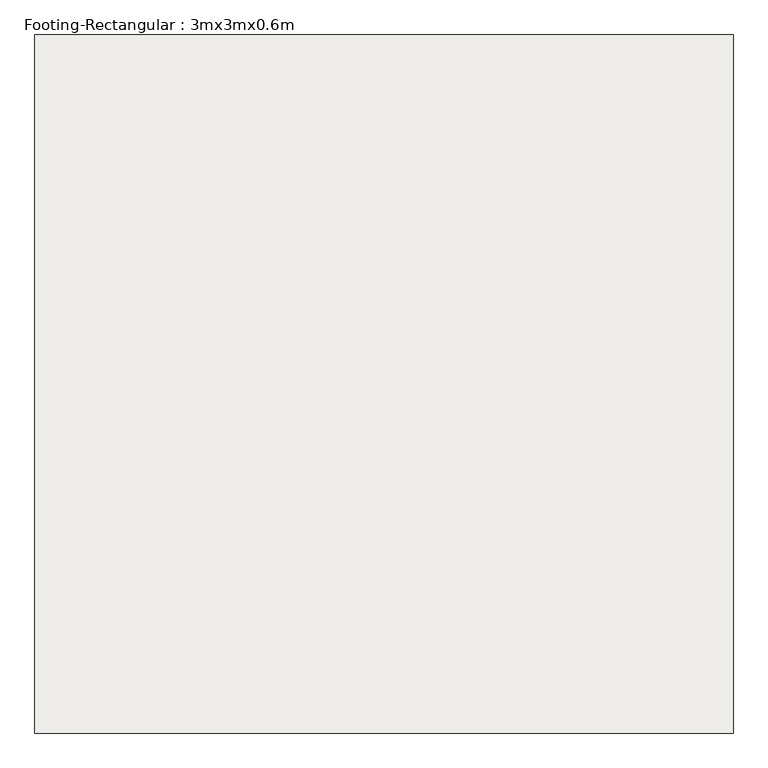
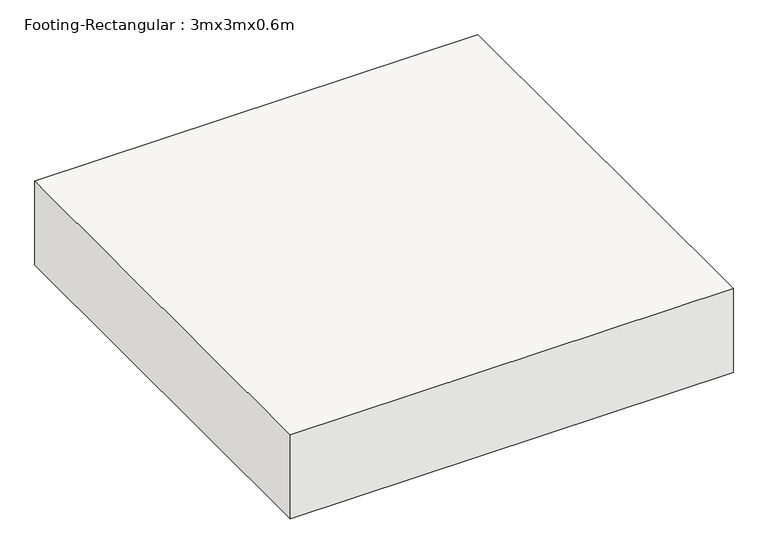
"""IFC4 building model written with IfcOpenShell, lengths in millimetres: slab geometry, Footing-Rectangular : 3mx3mx0.6m."""

from ifc_helpers import new_model, si_unit, frame, origin, place, context, project, spatial, polyline, outline, extrude, source, transform, mapped, element, save


def footing_rectangular_3mx3mx0_6m_b12d3fe5(model_context):
    return source(origin(), model_context, "Body", "SweptSolid", [
        extrude(outline(polyline([(1499.9890625, 1499.9890625), (1499.9890625, -1499.9890625), (-1499.9890625, -1499.9890625), (-1499.9890625, 1499.9890625), (1499.9890625, 1499.9890625)])), frame((0.0, 0.0, -599.9757812), z_axis=(0.0, 0.0, 1.0), x_axis=(1.0, 0.0, 0.0)), (0.0, 0.0, 1.0), 599.9757812),
    ])


if __name__ == "__main__":
    model = new_model("IFC4")
    model_context = context("Model", 3, world=origin())
    ifc_project = project(units=[si_unit("LENGTHUNIT", "METRE", prefix="MILLI")], contexts=[model_context])
    site = spatial("IfcSite", under=ifc_project)
    building = spatial("IfcBuilding", under=site)
    placement = place(None, origin())
    footing_rectangular_3mx3mx0_6m_shape = footing_rectangular_3mx3mx0_6m_b12d3fe5(model_context)
    element("IfcSlab", 1, ObjectType="Footing-Rectangular : 3mx3mx0.6m", at=placement, inside=building, context=model_context, shape_type="MappedRepresentation", body=[
        mapped(footing_rectangular_3mx3mx0_6m_shape, transform((0.0, 0.0, 0.0), x_axis=(1.0, 0.0, 0.0), y_axis=(0.0, 1.0, 0.0), z_axis=(0.0, 0.0, 1.0))),
    ])
    save(model, "model.ifc")

# Revit data of these elements
# Type "Footing-Rectangular : 3mx3mx0.6m"
#   Width = 2999.978 mm
#   Length = 2999.978 mm
#   Foundation Thickness = 599.976 mm
#   Structural Material [instance default] = Concrete, Cast-in-Place gray
# Element 1 (IfcSlab, "Footing-Rectangular : 3mx3mx0.6m")
#   Materials on its faces: "Concrete, Cast-in-Place gray"
# Materials
#   "Concrete, Cast-in-Place gray": class "Concrete", colour RGB 192 192 192, transparency 0, Description = "Cast-in-place concrete", Cost = 0
